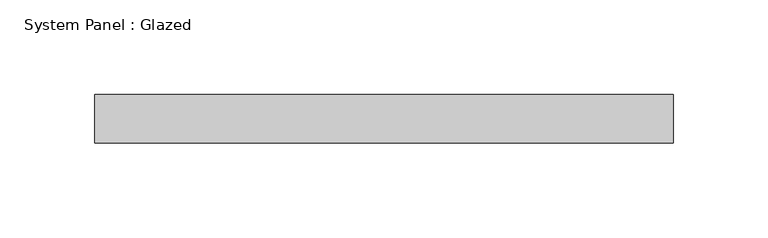
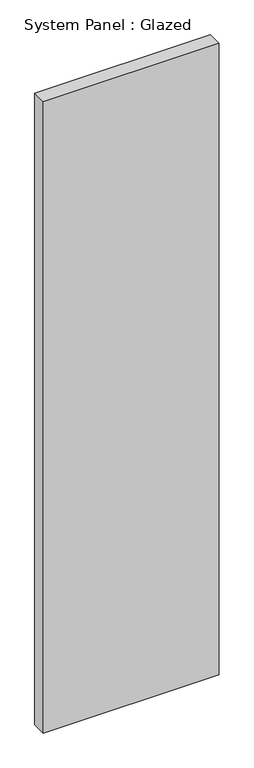
"""IFC4 building model written with IfcOpenShell, lengths in millimetres: plate geometry, System Panel : Glazed."""

from ifc_helpers import new_model, si_unit, origin, origin_with_axes, place, context, project, spatial, polyline, outline, extrude, source, transform, mapped, element, save


def system_panel_glazed_1fa29e7b(model_context):
    return source(origin(), model_context, "Body", "SweptSolid", [
        extrude(outline(polyline([(152.4, 19.05), (-152.4, 19.05), (-152.4, 44.45), (152.4, 44.45), (152.4, 19.05)])), origin_with_axes(), (0.0, 0.0, 1.0), 1155.7),
    ])


if __name__ == "__main__":
    model = new_model("IFC4")
    model_context = context("Model", 3, world=origin())
    ifc_project = project(units=[si_unit("LENGTHUNIT", "METRE", prefix="MILLI")], contexts=[model_context])
    site = spatial("IfcSite", under=ifc_project)
    building = spatial("IfcBuilding", under=site)
    placement = place(None, origin())
    system_panel_glazed_shape = system_panel_glazed_1fa29e7b(model_context)
    element("IfcPlate", 1, ObjectType="System Panel : Glazed", at=placement, inside=building, context=model_context, shape_type="MappedRepresentation", body=[
        mapped(system_panel_glazed_shape, transform((0.0, 0.0, 0.0), x_axis=(1.0, 0.0, 0.0), y_axis=(0.0, 1.0, 0.0), z_axis=(0.0, 0.0, 1.0))),
    ])
    save(model, "model.ifc")

# Revit data of these elements
# Type "System Panel : Glazed"
#   Construction Type Id = "GSP4R"
#   Analytic Construction = "1/8 in Pilkington single glazing"
#   Visual Light Transmittance = 0.9
#   Solar Heat Gain Coefficient = 0.86
#   Heat Transfer Coefficient (U) = 1.18115 BTU/(h·ft²·°F)
# Element 1 (IfcPlate, "System Panel : Glazed")
#   Materials on its faces: "Glass"
# Materials
#   "Glass": class "Glass", colour RGB 0 128 192, transparency 0.75, Description = "Soda Lime Glass", Cost = 0
